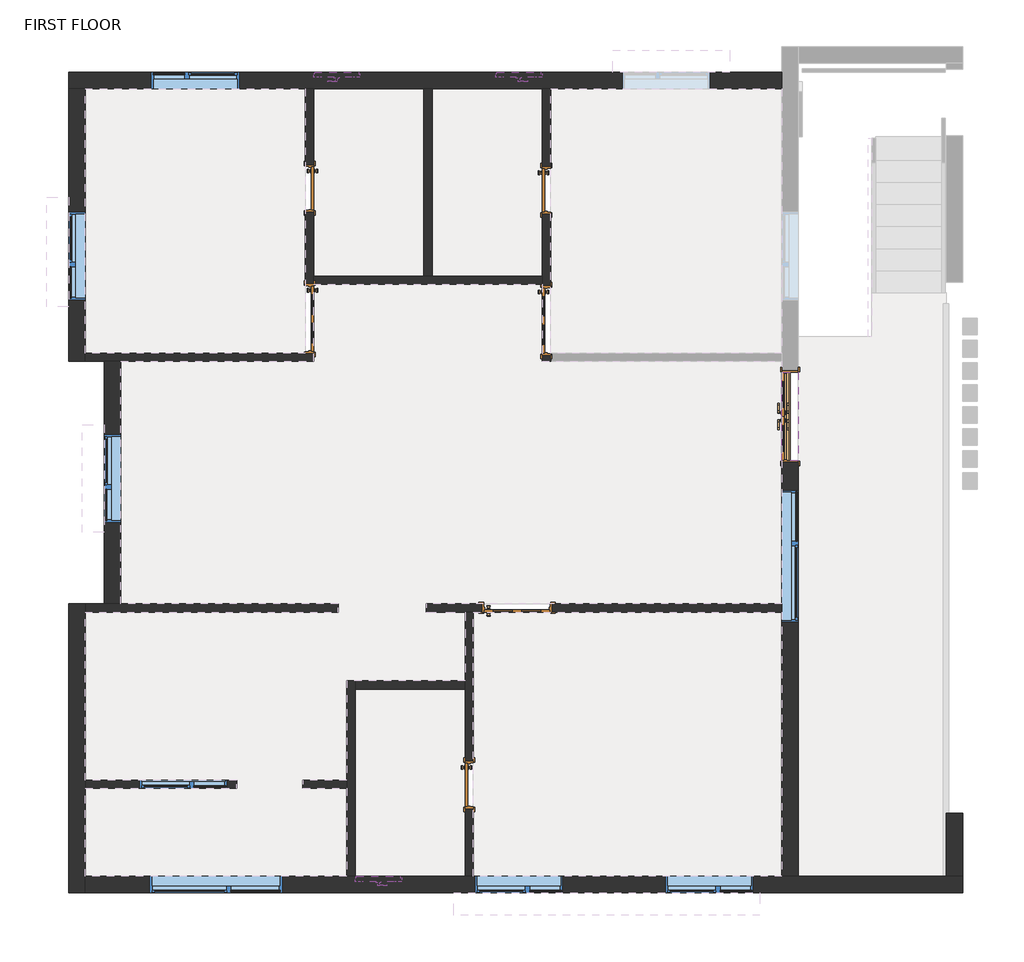
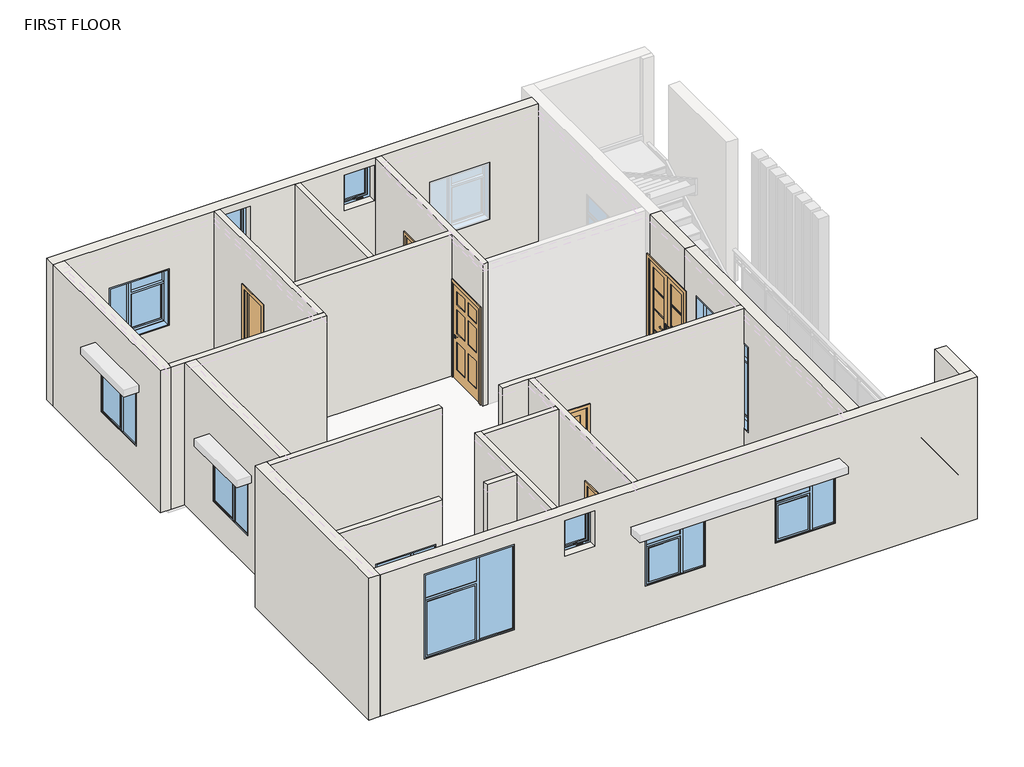
# One storey, part 1 of 2: 20 walls, 11 windows, 7 doors.
"""IFC4 building model written with IfcOpenShell, lengths in millimetres."""

from ifc_helpers import new_model, si_unit, frame, origin, place, context, project, spatial, polyline, outline, extrude, faceted_brep, transform, mapped, element, save
from components import door_exterior_double_full_glass_wood_clad_double_main_door_4_3788f36b, door_92bad2d9, door_a4da38fb, door_0e119d28, door_525aa856, window_610_x_762_5077743b, window_610_x_762_22856471, window_casement_double_sidelight_window_4_x_4_2a492e8f, window_casement_double_sidelight_window_4_x_4_ae1e99d1, window_casement_double_sidelight_window_6_x_6_6a7c62ef

model = new_model("IFC4")

# Units and contexts
model_context = context("Model", 3, world=origin())
ifc_project = project(units=[si_unit("LENGTHUNIT", "METRE", prefix="MILLI")], contexts=[model_context])

# Site, building, storey
site = spatial("IfcSite", under=ifc_project)
building = spatial("IfcBuilding", under=site)
storey = spatial("IfcBuildingStorey", under=building, Name="FIRST FLOOR", Elevation=3048.0)

# Doors
placement = place(None, origin())
door_exterior_double_full_glass_wood_clad_double_main_door_4_shape = door_exterior_double_full_glass_wood_clad_double_main_door_4_3788f36b(model_context)
element("IfcDoor", 1, ObjectType="Door-Exterior-Double-Full Glass-Wood_Clad : double main door 4' x 7'", at=placement, inside=storey, context=model_context, shape_type="MappedRepresentation", body=[
    mapped(door_exterior_double_full_glass_wood_clad_double_main_door_4_shape, transform((-4646.5406154, 1972.1500875, 3022.6), x_axis=(0.0, 1.0, 0.0), y_axis=(-1.0, 0.0, 0.0), z_axis=(0.0, 0.0, 1.0))),
])
door_shape = door_92bad2d9(model_context)
element("IfcDoor", 2, ObjectType="Door-Interior-Single-6_Panel-Wood : 36\" x 80\"", at=placement, inside=storey, context=model_context, shape_type="MappedRepresentation", body=[
    mapped(door_shape, transform((-11288.6406154, 3324.7000875, 3048.0), x_axis=(0.0, -1.0, 0.0), y_axis=(1.0, 0.0, 0.0), z_axis=(0.0, 0.0, 1.0))),
])
door_2_shape = door_a4da38fb(model_context)
element("IfcDoor", 3, ObjectType="Door-Interior-Single-6_Panel-Wood : 36\" x 80\"", at=placement, inside=storey, context=model_context, shape_type="MappedRepresentation", body=[
    mapped(door_2_shape, transform((-8018.3906154, 3299.3000875, 3048.0), x_axis=(0.0, -1.0, 0.0), y_axis=(1.0, 0.0, 0.0), z_axis=(0.0, 0.0, 1.0))),
])
element("IfcDoor", 4, ObjectType="Door-Interior-Single-6_Panel-Wood : 36\" x 80\"", at=placement, inside=storey, context=model_context, shape_type="MappedRepresentation", body=[
    mapped(door_2_shape, transform((-8421.6156154, -678.9749125, 3048.0), x_axis=(1.0, 0.0, 0.0), y_axis=(0.0, 1.0, 0.0), z_axis=(0.0, 0.0, 1.0))),
])
door_3_shape = door_0e119d28(model_context)
element("IfcDoor", 5, ObjectType="Door-Interior-Single-Flush_Panel-Wood : 24\" x 80\"", at=placement, inside=storey, context=model_context, shape_type="MappedRepresentation", body=[
    mapped(door_3_shape, transform((-11288.6406154, 5128.1000875, 3048.0), x_axis=(0.0, -1.0, 0.0), y_axis=(1.0, 0.0, 0.0), z_axis=(0.0, 0.0, 1.0))),
])
door_4_shape = door_525aa856(model_context)
element("IfcDoor", 6, ObjectType="Door-Interior-Single-Flush_Panel-Wood : 24\" x 80\"", at=placement, inside=storey, context=model_context, shape_type="MappedRepresentation", body=[
    mapped(door_4_shape, transform((-8018.3906154, 5102.7000875, 3048.0), x_axis=(0.0, -1.0, 0.0), y_axis=(1.0, 0.0, 0.0), z_axis=(0.0, 0.0, 1.0))),
])
element("IfcDoor", 7, ObjectType="Door-Interior-Single-Flush_Panel-Wood : 24\" x 80\"", at=placement, inside=storey, context=model_context, shape_type="MappedRepresentation", body=[
    mapped(door_4_shape, transform((-9085.1906154, -3123.7249125, 3048.0), x_axis=(0.0, -1.0, 0.0), y_axis=(1.0, 0.0, 0.0), z_axis=(0.0, 0.0, 1.0))),
])

# Walls
element("IfcWall", 8, at=placement, inside=storey, context=model_context, shape_type="Brep", body=[
    faceted_brep([(-4757.6656154, 6734.6500875, 3048.0), (-14625.5656154, 6734.6500875, 3048.0), (-14625.5656154, 6734.6500875, 6096.0), (-4757.6656154, 6734.6500875, 6096.0), (-10612.3656154, 6734.6500875, 5181.6), (-10612.3656154, 6734.6500875, 5943.6), (-11221.9656154, 6734.6500875, 5943.6), (-11221.9656154, 6734.6500875, 5181.6), (-8701.0156154, 6734.6500875, 5943.6), (-8701.0156154, 6734.6500875, 5181.6), (-8091.4156154, 6734.6500875, 5181.6), (-8091.4156154, 6734.6500875, 5943.6), (-5748.2656154, 6734.6500875, 5181.6), (-6967.4656154, 6734.6500875, 5181.6), (-6967.4656154, 6734.6500875, 3962.4), (-5748.2656154, 6734.6500875, 3962.4), (-12263.3656154, 6734.6500875, 5181.6), (-13482.5656154, 6734.6500875, 5181.6), (-13482.5656154, 6734.6500875, 3962.4), (-12263.3656154, 6734.6500875, 3962.4), (-4757.6656154, 6506.0500875, 3048.0), (-4757.6656154, 6506.0500875, 6096.0), (-7958.0656154, 6506.0500875, 6096.0), (-8072.3656154, 6506.0500875, 6096.0), (-9596.3656154, 6506.0500875, 6096.0), (-9710.6656154, 6506.0500875, 6096.0), (-11234.6656154, 6506.0500875, 6096.0), (-11348.9656154, 6506.0500875, 6096.0), (-14396.9656154, 6506.0500875, 6096.0), (-14625.5656154, 6506.0500875, 6096.0), (-14625.5656154, 6506.0500875, 3048.0), (-14396.9656154, 6506.0500875, 3048.0), (-11348.9656154, 6506.0500875, 3048.0), (-11234.6656154, 6506.0500875, 3048.0), (-9710.6656154, 6506.0500875, 3048.0), (-9596.3656154, 6506.0500875, 3048.0), (-8072.3656154, 6506.0500875, 3048.0), (-7958.0656154, 6506.0500875, 3048.0), (-10612.3656154, 6506.0500875, 5943.6), (-10612.3656154, 6506.0500875, 5181.6), (-11221.9656154, 6506.0500875, 5181.6), (-11221.9656154, 6506.0500875, 5943.6), (-8701.0156154, 6506.0500875, 5181.6), (-8701.0156154, 6506.0500875, 5943.6), (-8091.4156154, 6506.0500875, 5943.6), (-8091.4156154, 6506.0500875, 5181.6), (-5748.2656154, 6506.0500875, 5181.6), (-5748.2656154, 6506.0500875, 3962.4), (-6967.4656154, 6506.0500875, 3962.4), (-6967.4656154, 6506.0500875, 5181.6), (-12263.3656154, 6506.0500875, 5181.6), (-12263.3656154, 6506.0500875, 3962.4), (-13482.5656154, 6506.0500875, 3962.4), (-13482.5656154, 6506.0500875, 5181.6)], [[[0, 1, 2, 3], [4, 5, 6, 7], [8, 9, 10, 11], [12, 13, 14, 15], [16, 17, 18, 19]], [[20, 21, 22, 23, 24, 25, 26, 27, 28, 29, 30, 31, 32, 33, 34, 35, 36, 37], [38, 39, 40, 41], [42, 43, 44, 45], [46, 47, 48, 49], [50, 51, 52, 53]], [[1, 0, 20, 37, 36, 35, 34, 33, 32, 31, 30]], [[3, 2, 29, 28, 27, 26, 25, 24, 23, 22, 21]], [[2, 1, 30, 29]], [[39, 38, 5, 4]], [[4, 7, 40, 39]], [[7, 6, 41, 40]], [[38, 41, 6, 5]], [[42, 9, 8, 43]], [[9, 42, 45, 10]], [[10, 45, 44, 11]], [[43, 8, 11, 44]], [[47, 46, 12, 15]], [[48, 47, 15, 14]], [[49, 48, 14, 13]], [[46, 49, 13, 12]], [[51, 50, 16, 19]], [[52, 51, 19, 18]], [[53, 52, 18, 17]], [[50, 53, 17, 16]], [[0, 3, 21, 20]]]),
])
element("IfcWall", 9, at=placement, inside=storey, context=model_context, shape_type="Brep", body=[
    faceted_brep([(-14625.5656154, 6506.0500875, 3048.0), (-14625.5656154, 2734.1500875, 3048.0), (-14625.5656154, 2734.1500875, 6096.0), (-14625.5656154, 6506.0500875, 6096.0), (-14625.5656154, 4803.1295492, 5181.6), (-14625.5656154, 3583.9295492, 5181.6), (-14625.5656154, 3583.9295492, 3962.4), (-14625.5656154, 4803.1295492, 3962.4), (-14396.9656154, 6506.0500875, 3048.0), (-14396.9656154, 6506.0500875, 6096.0), (-14396.9656154, 2848.4500875, 6096.0), (-14396.9656154, 2734.1500875, 6096.0), (-14396.9656154, 2734.1500875, 3048.0), (-14396.9656154, 2848.4500875, 3048.0), (-14396.9656154, 4803.1295492, 5181.6), (-14396.9656154, 4803.1295492, 3962.4), (-14396.9656154, 3583.9295492, 3962.4), (-14396.9656154, 3583.9295492, 5181.6)], [[[0, 1, 2, 3], [4, 5, 6, 7]], [[8, 9, 10, 11, 12, 13], [14, 15, 16, 17]], [[1, 0, 8, 13, 12]], [[3, 2, 11, 10, 9]], [[0, 3, 9, 8]], [[2, 1, 12, 11]], [[15, 14, 4, 7]], [[16, 15, 7, 6]], [[17, 16, 6, 5]], [[14, 17, 5, 4]]]),
])
element("IfcWall", 10, at=placement, inside=storey, context=model_context, shape_type="Brep", body=[
    faceted_brep([(-14625.5656154, -618.6499125, 3048.0), (-14625.5656154, -4619.1499125, 3048.0), (-14625.5656154, -4619.1499125, 6096.0), (-14625.5656154, -618.6499125, 6096.0), (-14396.9656154, -618.6499125, 3048.0), (-14396.9656154, -618.6499125, 6096.0), (-14396.9656154, -732.9499125, 6096.0), (-14396.9656154, -3057.0499125, 6096.0), (-14396.9656154, -3171.3499125, 6096.0), (-14396.9656154, -4390.5499125, 6096.0), (-14396.9656154, -4619.1499125, 6096.0), (-14396.9656154, -4619.1499125, 3048.0), (-14396.9656154, -4390.5499125, 3048.0), (-14396.9656154, -3171.3499125, 3048.0), (-14396.9656154, -3057.0499125, 3048.0), (-14396.9656154, -732.9499125, 3048.0)], [[[0, 1, 2, 3]], [[4, 5, 6, 7, 8, 9, 10, 11, 12, 13, 14, 15]], [[1, 0, 4, 15, 14, 13, 12, 11]], [[3, 2, 10, 9, 8, 7, 6, 5]], [[2, 1, 11, 10]], [[0, 3, 5, 4]]]),
])
element("IfcWall", 11, at=placement, inside=storey, context=model_context, shape_type="Brep", body=[
    faceted_brep([(-14396.9656154, -4619.1499125, 3048.0), (-2255.7656154, -4619.1499125, 3048.0), (-2255.7656154, -4619.1499125, 6096.0), (-14396.9656154, -4619.1499125, 6096.0), (-10644.1156154, -4619.1499125, 5181.6), (-10644.1156154, -4619.1499125, 5943.6), (-10034.5156154, -4619.1499125, 5943.6), (-10034.5156154, -4619.1499125, 5181.6), (-9005.8156154, -4619.1499125, 5181.6), (-7786.6156154, -4619.1499125, 5181.6), (-7786.6156154, -4619.1499125, 3962.4), (-9005.8156154, -4619.1499125, 3962.4), (-6370.5656154, -4619.1499125, 5181.6), (-5151.3656154, -4619.1499125, 5181.6), (-5151.3656154, -4619.1499125, 3962.4), (-6370.5656154, -4619.1499125, 3962.4), (-13501.6156154, -4619.1499125, 5791.2), (-11672.8156154, -4619.1499125, 5791.2), (-11672.8156154, -4619.1499125, 3962.4), (-13501.6156154, -4619.1499125, 3962.4), (-14396.9656154, -4390.5499125, 3048.0), (-14396.9656154, -4390.5499125, 6096.0), (-10777.4656154, -4390.5499125, 6096.0), (-10663.1656154, -4390.5499125, 6096.0), (-9139.1656154, -4390.5499125, 6096.0), (-9024.8656154, -4390.5499125, 6096.0), (-4757.6656154, -4390.5499125, 6096.0), (-4529.0656154, -4390.5499125, 6096.0), (-2484.3656154, -4390.5499125, 6096.0), (-2255.7656154, -4390.5499125, 6096.0), (-2255.7656154, -4390.5499125, 3048.0), (-2484.3656154, -4390.5499125, 3048.0), (-4529.0656154, -4390.5499125, 3048.0), (-4757.6656154, -4390.5499125, 3048.0), (-9024.8656154, -4390.5499125, 3048.0), (-9139.1656154, -4390.5499125, 3048.0), (-10663.1656154, -4390.5499125, 3048.0), (-10777.4656154, -4390.5499125, 3048.0), (-10644.1156154, -4390.5499125, 5943.6), (-10644.1156154, -4390.5499125, 5181.6), (-10034.5156154, -4390.5499125, 5181.6), (-10034.5156154, -4390.5499125, 5943.6), (-9005.8156154, -4390.5499125, 5181.6), (-9005.8156154, -4390.5499125, 3962.4), (-7786.6156154, -4390.5499125, 3962.4), (-7786.6156154, -4390.5499125, 5181.6), (-6370.5656154, -4390.5499125, 5181.6), (-6370.5656154, -4390.5499125, 3962.4), (-5151.3656154, -4390.5499125, 3962.4), (-5151.3656154, -4390.5499125, 5181.6), (-13501.6156154, -4390.5499125, 5791.2), (-13501.6156154, -4390.5499125, 3962.4), (-11672.8156154, -4390.5499125, 3962.4), (-11672.8156154, -4390.5499125, 5791.2)], [[[0, 1, 2, 3], [4, 5, 6, 7], [8, 9, 10, 11], [12, 13, 14, 15], [16, 17, 18, 19]], [[20, 21, 22, 23, 24, 25, 26, 27, 28, 29, 30, 31, 32, 33, 34, 35, 36, 37], [38, 39, 40, 41], [42, 43, 44, 45], [46, 47, 48, 49], [50, 51, 52, 53]], [[1, 0, 20, 37, 36, 35, 34, 33, 32, 31, 30]], [[3, 2, 29, 28, 27, 26, 25, 24, 23, 22, 21]], [[0, 3, 21, 20]], [[4, 39, 38, 5]], [[39, 4, 7, 40]], [[40, 7, 6, 41]], [[5, 38, 41, 6]], [[43, 42, 8, 11]], [[44, 43, 11, 10]], [[45, 44, 10, 9]], [[42, 45, 9, 8]], [[47, 46, 12, 15]], [[48, 47, 15, 14]], [[49, 48, 14, 13]], [[46, 49, 13, 12]], [[51, 50, 16, 19]], [[52, 51, 19, 18]], [[53, 52, 18, 17]], [[50, 53, 17, 16]], [[2, 1, 30, 29]]]),
])
element("IfcWall", 12, at=placement, inside=storey, context=model_context, shape_type="Brep", body=[
    faceted_brep([(-4529.0656154, 1362.5500875, 6096.0), (-4529.0656154, -4390.5499125, 6096.0), (-4529.0656154, -4390.5499125, 3048.0), (-4529.0656154, 1337.1500875, 3048.0), (-4529.0656154, 1337.1500875, 5181.6), (-4529.0656154, 1362.5500875, 5181.6), (-4529.0656154, -875.0434232, 5334.0), (-4529.0656154, 953.7565768, 5334.0), (-4529.0656154, 953.7565768, 3505.2), (-4529.0656154, -875.0434232, 3505.2), (-4757.6656154, -4390.5499125, 6096.0), (-4757.6656154, -732.9499125, 6096.0), (-4757.6656154, -618.6499125, 6096.0), (-4757.6656154, 1362.5500875, 6096.0), (-4757.6656154, 1362.5500875, 5181.6), (-4757.6656154, 1337.1500875, 5181.6), (-4757.6656154, 1337.1500875, 3048.0), (-4757.6656154, -618.6499125, 3048.0), (-4757.6656154, -732.9499125, 3048.0), (-4757.6656154, -4390.5499125, 3048.0), (-4757.6656154, -875.0434232, 5334.0), (-4757.6656154, -875.0434232, 3505.2), (-4757.6656154, 953.7565768, 3505.2), (-4757.6656154, 953.7565768, 5334.0)], [[[0, 1, 2, 3, 4, 5], [6, 7, 8, 9]], [[10, 11, 12, 13, 14, 15, 16, 17, 18, 19], [20, 21, 22, 23]], [[2, 19, 18, 17, 16, 3]], [[13, 0, 5, 14]], [[1, 0, 13, 12, 11, 10]], [[2, 1, 10, 19]], [[4, 15, 14, 5]], [[15, 4, 3, 16]], [[21, 20, 6, 9]], [[22, 21, 9, 8]], [[23, 22, 8, 7]], [[20, 23, 7, 6]]]),
])
element("IfcWall", 13, at=placement, inside=storey, context=model_context, shape_type="Brep", body=[
    faceted_brep([(-14396.9656154, -732.9499125, 3048.0), (-10895.4913348, -732.9499125, 3048.0), (-10895.4913348, -732.9499125, 6096.0), (-14396.9656154, -732.9499125, 6096.0), (-14396.9656154, -618.6499125, 3048.0), (-14396.9656154, -618.6499125, 6096.0), (-14130.2656154, -618.6499125, 6096.0), (-13901.6656154, -618.6499125, 6096.0), (-10895.4913348, -618.6499125, 6096.0), (-10895.4913348, -618.6499125, 3048.0), (-13901.6656154, -618.6499125, 3048.0), (-14130.2656154, -618.6499125, 3048.0)], [[[0, 1, 2, 3]], [[4, 5, 6, 7, 8, 9, 10, 11]], [[1, 0, 4, 11, 10, 9]], [[2, 1, 9, 8]], [[3, 2, 8, 7, 6, 5]], [[0, 3, 5, 4]]]),
])
element("IfcWall", 14, at=placement, inside=storey, context=model_context, shape_type="SweptSolid", body=[
    extrude(outline(polyline([(3048.0, -14396.9656154), (3048.0, -12301.4656154), (6096.0, -12301.4656154), (6096.0, -14396.9656154), (3048.0, -14396.9656154)]), holes=[polyline([(5181.6, -13647.6656154), (5181.6, -12428.4656154), (3962.4, -12428.4656154), (3962.4, -13647.6656154), (5181.6, -13647.6656154)])]), frame((0.0, -3171.3499125, 0.0), z_axis=(0.0, 1.0, 0.0), x_axis=(0.0, 0.0, 1.0)), (0.0, 0.0, 1.0), 114.3),
])
element("IfcWall", 15, at=placement, inside=storey, context=model_context, shape_type="SweptSolid", body=[
    extrude(outline(polyline([(-11387.0656154, -3057.0499125), (-10777.4656154, -3057.0499125), (-10777.4656154, -3171.3499125), (-11387.0656154, -3171.3499125), (-11387.0656154, -3057.0499125)])), frame((0.0, 0.0, 3048.0), z_axis=(0.0, 0.0, 1.0), x_axis=(1.0, 0.0, 0.0)), (0.0, 0.0, 1.0), 3048.0),
])
element("IfcWall", 16, at=placement, inside=storey, context=model_context, shape_type="Brep", body=[
    faceted_brep([(-10663.1656154, -4390.5499125, 3048.0), (-10663.1656154, -1799.7499125, 3048.0), (-10663.1656154, -1685.4499125, 3048.0), (-10663.1656154, -1685.4499125, 6096.0), (-10663.1656154, -1799.7499125, 6096.0), (-10663.1656154, -4390.5499125, 6096.0), (-10777.4656154, -4390.5499125, 3048.0), (-10777.4656154, -4390.5499125, 6096.0), (-10777.4656154, -3171.3499125, 6096.0), (-10777.4656154, -3057.0499125, 6096.0), (-10777.4656154, -1685.4499125, 6096.0), (-10777.4656154, -1685.4499125, 3048.0), (-10777.4656154, -3057.0499125, 3048.0), (-10777.4656154, -3171.3499125, 3048.0)], [[[0, 1, 2, 3, 4, 5]], [[6, 7, 8, 9, 10, 11, 12, 13]], [[2, 1, 0, 6, 13, 12, 11]], [[5, 4, 3, 10, 9, 8, 7]], [[0, 5, 7, 6]], [[3, 2, 11, 10]]]),
])
element("IfcWall", 17, at=placement, inside=storey, context=model_context, shape_type="SweptSolid", body=[
    extrude(outline(polyline([(-9139.1656154, -1799.7499125), (-10663.1656154, -1799.7499125), (-10663.1656154, -1685.4499125), (-9139.1656154, -1685.4499125), (-9139.1656154, -1799.7499125)])), frame((0.0, 0.0, 3048.0), z_axis=(0.0, 0.0, 1.0), x_axis=(1.0, 0.0, 0.0)), (0.0, 0.0, 1.0), 3048.0),
])
element("IfcWall", 18, at=placement, inside=storey, context=model_context, shape_type="Brep", body=[
    faceted_brep([(-9024.8656154, -732.9499125, 6096.0), (-9024.8656154, -4390.5499125, 6096.0), (-9024.8656154, -4390.5499125, 3048.0), (-9024.8656154, -3453.9249125, 3048.0), (-9024.8656154, -3453.9249125, 5105.4), (-9024.8656154, -2793.5249125, 5105.4), (-9024.8656154, -2793.5249125, 3048.0), (-9024.8656154, -732.9499125, 3048.0), (-9139.1656154, -4390.5499125, 6096.0), (-9139.1656154, -1799.7499125, 6096.0), (-9139.1656154, -1685.4499125, 6096.0), (-9139.1656154, -732.9499125, 6096.0), (-9139.1656154, -732.9499125, 3048.0), (-9139.1656154, -1685.4499125, 3048.0), (-9139.1656154, -1799.7499125, 3048.0), (-9139.1656154, -2793.5249125, 3048.0), (-9139.1656154, -2793.5249125, 5105.4), (-9139.1656154, -3453.9249125, 5105.4), (-9139.1656154, -3453.9249125, 3048.0), (-9139.1656154, -4390.5499125, 3048.0)], [[[0, 1, 2, 3, 4, 5, 6, 7]], [[8, 9, 10, 11, 12, 13, 14, 15, 16, 17, 18, 19]], [[12, 7, 6, 15, 14, 13]], [[2, 19, 18, 3]], [[1, 0, 11, 10, 9, 8]], [[0, 7, 12, 11]], [[2, 1, 8, 19]], [[17, 4, 3, 18]], [[4, 17, 16, 5]], [[5, 16, 15, 6]]]),
])
element("IfcWall", 19, at=placement, inside=storey, context=model_context, shape_type="Brep", body=[
    faceted_brep([(-8072.3656154, 2734.1500875, 6096.0), (-8072.3656154, 3800.9500875, 6096.0), (-8072.3656154, 3915.2500875, 6096.0), (-8072.3656154, 6506.0500875, 6096.0), (-8072.3656154, 6506.0500875, 3048.0), (-8072.3656154, 5432.9000875, 3048.0), (-8072.3656154, 5432.9000875, 5105.4), (-8072.3656154, 4772.5000875, 5105.4), (-8072.3656154, 4772.5000875, 3048.0), (-8072.3656154, 3915.2500875, 3048.0), (-8072.3656154, 3800.9500875, 3048.0), (-8072.3656154, 3781.9000875, 3048.0), (-8072.3656154, 3781.9000875, 5105.4), (-8072.3656154, 2816.7000875, 5105.4), (-8072.3656154, 2816.7000875, 3048.0), (-8072.3656154, 2734.1500875, 3048.0), (-7958.0656154, 6506.0500875, 6096.0), (-7958.0656154, 2848.4500875, 6096.0), (-7958.0656154, 2734.1500875, 6096.0), (-7958.0656154, 2734.1500875, 3048.0), (-7958.0656154, 2816.7000875, 3048.0), (-7958.0656154, 2816.7000875, 5105.4), (-7958.0656154, 3781.9000875, 5105.4), (-7958.0656154, 3781.9000875, 3048.0), (-7958.0656154, 4772.5000875, 3048.0), (-7958.0656154, 4772.5000875, 5105.4), (-7958.0656154, 5432.9000875, 5105.4), (-7958.0656154, 5432.9000875, 3048.0), (-7958.0656154, 6506.0500875, 3048.0)], [[[0, 1, 2, 3, 4, 5, 6, 7, 8, 9, 10, 11, 12, 13, 14, 15]], [[16, 17, 18, 19, 20, 21, 22, 23, 24, 25, 26, 27, 28]], [[4, 28, 27, 5]], [[19, 15, 14, 20]], [[23, 11, 10, 9, 8, 24]], [[3, 2, 1, 0, 18, 17, 16]], [[4, 3, 16, 28]], [[0, 15, 19, 18]], [[14, 13, 21, 20]], [[13, 12, 22, 21]], [[12, 11, 23, 22]], [[7, 25, 24, 8]], [[25, 7, 6, 26]], [[26, 6, 5, 27]]]),
])
element("IfcWall", 20, at=placement, inside=storey, context=model_context, shape_type="Brep", body=[
    faceted_brep([(-8072.3656154, 3915.2500875, 3048.0), (-9596.3656154, 3915.2500875, 3048.0), (-9710.6656154, 3915.2500875, 3048.0), (-11234.6656154, 3915.2500875, 3048.0), (-11234.6656154, 3915.2500875, 6096.0), (-9710.6656154, 3915.2500875, 6096.0), (-9596.3656154, 3915.2500875, 6096.0), (-8072.3656154, 3915.2500875, 6096.0), (-8072.3656154, 3800.9500875, 3048.0), (-8072.3656154, 3800.9500875, 6096.0), (-11234.6656154, 3800.9500875, 6096.0), (-11234.6656154, 3800.9500875, 3048.0), (-11234.6656154, 3807.3000875, 3048.0)], [[[0, 1, 2, 3, 4, 5, 6, 7]], [[8, 9, 10, 11]], [[3, 2, 1, 0, 8, 11, 12]], [[7, 6, 5, 4, 10, 9]], [[0, 7, 9, 8]], [[4, 3, 12, 11, 10]]]),
])
element("IfcWall", 21, at=placement, inside=storey, context=model_context, shape_type="Brep", body=[
    faceted_brep([(-11234.6656154, 6506.0500875, 6096.0), (-11234.6656154, 3915.2500875, 6096.0), (-11234.6656154, 3800.9500875, 6096.0), (-11234.6656154, 2848.4500875, 6096.0), (-11234.6656154, 2848.4500875, 5105.4), (-11234.6656154, 3807.3000875, 5105.4), (-11234.6656154, 3807.3000875, 3048.0), (-11234.6656154, 3915.2500875, 3048.0), (-11234.6656154, 4797.9000875, 3048.0), (-11234.6656154, 4797.9000875, 5105.4), (-11234.6656154, 5458.3000875, 5105.4), (-11234.6656154, 5458.3000875, 3048.0), (-11234.6656154, 6506.0500875, 3048.0), (-11348.9656154, 2848.4500875, 6096.0), (-11348.9656154, 6506.0500875, 6096.0), (-11348.9656154, 6506.0500875, 3048.0), (-11348.9656154, 5458.3000875, 3048.0), (-11348.9656154, 5458.3000875, 5105.4), (-11348.9656154, 4797.9000875, 5105.4), (-11348.9656154, 4797.9000875, 3048.0), (-11348.9656154, 3807.3000875, 3048.0), (-11348.9656154, 3807.3000875, 5105.4), (-11348.9656154, 2848.4500875, 5105.4)], [[[0, 1, 2, 3, 4, 5, 6, 7, 8, 9, 10, 11, 12]], [[13, 14, 15, 16, 17, 18, 19, 20, 21, 22]], [[15, 12, 11, 16]], [[6, 20, 19, 8, 7]], [[3, 2, 1, 0, 14, 13]], [[0, 12, 15, 14]], [[3, 13, 22, 4]], [[21, 5, 4, 22]], [[5, 21, 20, 6]], [[18, 9, 8, 19]], [[9, 18, 17, 10]], [[10, 17, 16, 11]]]),
])
element("IfcWall", 22, at=placement, inside=storey, context=model_context, shape_type="SweptSolid", body=[
    extrude(outline(polyline([(-9710.6656154, 3915.2500875), (-9710.6656154, 6506.0500875), (-9596.3656154, 6506.0500875), (-9596.3656154, 3915.2500875), (-9710.6656154, 3915.2500875)])), frame((0.0, 0.0, 3048.0), z_axis=(0.0, 0.0, 1.0), x_axis=(1.0, 0.0, 0.0)), (0.0, 0.0, 1.0), 3048.0),
])
element("IfcWall", 23, at=placement, inside=storey, context=model_context, shape_type="Brep", body=[
    faceted_brep([(-14396.9656154, 2734.1500875, 3048.0), (-14130.2656154, 2734.1500875, 3048.0), (-13901.6656154, 2734.1500875, 3048.0), (-11234.6656154, 2734.1500875, 3048.0), (-11234.6656154, 2734.1500875, 6096.0), (-13901.6656154, 2734.1500875, 6096.0), (-14130.2656154, 2734.1500875, 6096.0), (-14396.9656154, 2734.1500875, 6096.0), (-14396.9656154, 2848.4500875, 6096.0), (-11348.9656154, 2848.4500875, 6096.0), (-11234.6656154, 2848.4500875, 6096.0), (-11234.6656154, 2848.4500875, 5105.4), (-11348.9656154, 2848.4500875, 5105.4), (-11348.9656154, 2848.4500875, 3048.0), (-14396.9656154, 2848.4500875, 3048.0), (-11348.9656154, 2842.1000875, 3048.0), (-11234.6656154, 2842.1000875, 3048.0), (-11234.6656154, 2842.1000875, 5105.4), (-11348.9656154, 2842.1000875, 5105.4)], [[[0, 1, 2, 3, 4, 5, 6, 7]], [[8, 9, 10, 11, 12, 13, 14]], [[3, 2, 1, 0, 14, 13, 15, 16]], [[7, 6, 5, 4, 10, 9, 8]], [[0, 7, 8, 14]], [[4, 3, 16, 17, 11, 10]], [[18, 15, 13, 12]], [[15, 18, 17, 16]], [[17, 18, 12, 11]]]),
])
element("IfcWall", 24, at=placement, inside=storey, context=model_context, shape_type="SweptSolid", body=[
    extrude(outline(polyline([(-4757.6656154, 1362.5500875), (-4757.6656154, 2581.7500875), (-4529.0656154, 2581.7500875), (-4529.0656154, 1362.5500875), (-4757.6656154, 1362.5500875)])), frame((0.0, 0.0, 5181.6), z_axis=(0.0, 0.0, 1.0), x_axis=(1.0, 0.0, 0.0)), (0.0, 0.0, 1.0), 914.4),
])
element("IfcWall", 25, at=placement, inside=storey, context=model_context, shape_type="Brep", body=[
    faceted_brep([(-9676.2913348, -618.6499125, 3048.0), (-9676.2913348, -618.6499125, 6096.0), (-4757.6656154, -618.6499125, 6096.0), (-4757.6656154, -618.6499125, 3048.0), (-7939.0156154, -618.6499125, 3048.0), (-7939.0156154, -618.6499125, 5105.4), (-8904.2156154, -618.6499125, 5105.4), (-8904.2156154, -618.6499125, 3048.0), (-9676.2913348, -732.9499125, 6096.0), (-9676.2913348, -732.9499125, 3048.0), (-9139.1656154, -732.9499125, 3048.0), (-9024.8656154, -732.9499125, 3048.0), (-8904.2156154, -732.9499125, 3048.0), (-8904.2156154, -732.9499125, 5105.4), (-7939.0156154, -732.9499125, 5105.4), (-7939.0156154, -732.9499125, 3048.0), (-4757.6656154, -732.9499125, 3048.0), (-4757.6656154, -732.9499125, 6096.0), (-9024.8656154, -732.9499125, 6096.0), (-9139.1656154, -732.9499125, 6096.0)], [[[0, 1, 2, 3, 4, 5, 6, 7]], [[8, 9, 10, 11, 12, 13, 14, 15, 16, 17, 18, 19]], [[9, 0, 7, 12, 11, 10]], [[3, 16, 15, 4]], [[1, 0, 9, 8]], [[2, 1, 8, 19, 18, 17]], [[3, 2, 17, 16]], [[14, 5, 4, 15]], [[5, 14, 13, 6]], [[6, 13, 12, 7]]]),
])
element("IfcWall", 26, at=placement, inside=storey, context=model_context, shape_type="SweptSolid", body=[
    extrude(outline(polyline([(2734.1500875, 3048.0), (-618.6499125, 3048.0), (-618.6499125, 6096.0), (2734.1500875, 6096.0), (2734.1500875, 3048.0)]), holes=[polyline([(1724.5000875, 4948.6955341), (505.3000875, 4948.6955341), (505.3000875, 3729.4955341), (1724.5000875, 3729.4955341), (1724.5000875, 4948.6955341)])]), frame((-14130.2656154, 0.0, 0.0), z_axis=(1.0, 0.0, 0.0), x_axis=(0.0, 1.0, 0.0)), (0.0, 0.0, 1.0), 228.6),
])
element("IfcWall", 27, at=placement, inside=storey, context=model_context, shape_type="SweptSolid", body=[
    extrude(outline(polyline([(-2255.7656154, -3514.2499125), (-2255.7656154, -4390.5499125), (-2484.3656154, -4390.5499125), (-2484.3656154, -3514.2499125), (-2255.7656154, -3514.2499125)])), frame((0.0, 0.0, 3048.0), z_axis=(0.0, 0.0, 1.0), x_axis=(1.0, 0.0, 0.0)), (0.0, 0.0, 1.0), 3048.0),
])

# Windows
window_610_x_762_shape = window_610_x_762_5077743b(model_context)
element("IfcWindow", 28, ObjectType="610 x 762", at=placement, inside=storey, context=model_context, shape_type="MappedRepresentation", body=[
    mapped(window_610_x_762_shape, transform((-10917.1656154, 6620.3500875, 4381.6), x_axis=(-1.0, 0.0, 0.0), y_axis=(0.0, -1.0, 0.0), z_axis=(0.0, 0.0, 1.0))),
])
window_610_x_762_2_shape = window_610_x_762_22856471(model_context)
element("IfcWindow", 29, ObjectType="610 x 762", at=placement, inside=storey, context=model_context, shape_type="MappedRepresentation", body=[
    mapped(window_610_x_762_2_shape, transform((-8396.2156154, 6620.3500875, 4381.6), x_axis=(1.0, 0.0, 0.0), y_axis=(0.0, 1.0, 0.0), z_axis=(0.0, 0.0, 1.0))),
])
element("IfcWindow", 30, ObjectType="610 x 762", at=placement, inside=storey, context=model_context, shape_type="MappedRepresentation", body=[
    mapped(window_610_x_762_2_shape, transform((-10339.3156154, -4504.8499125, 4381.6), x_axis=(1.0, 0.0, 0.0), y_axis=(0.0, 1.0, 0.0), z_axis=(0.0, 0.0, 1.0))),
])
window_casement_double_sidelight_window_4_x_4_shape = window_casement_double_sidelight_window_4_x_4_2a492e8f(model_context)
element("IfcWindow", 31, ObjectType="Window-Casement-Double-Sidelight : window 4' x 4'", at=placement, inside=storey, context=model_context, shape_type="MappedRepresentation", body=[
    mapped(window_casement_double_sidelight_window_4_x_4_shape, transform((-8396.2156154, -4504.8499125, 3048.0), x_axis=(-1.0, 0.0, 0.0), y_axis=(0.0, -1.0, 0.0), z_axis=(0.0, 0.0, 1.0))),
])
element("IfcWindow", 32, ObjectType="Window-Casement-Double-Sidelight : window 4' x 4'", at=placement, inside=storey, context=model_context, shape_type="MappedRepresentation", body=[
    mapped(window_casement_double_sidelight_window_4_x_4_shape, transform((-5760.9656154, -4504.8499125, 3048.0), x_axis=(-1.0, 0.0, 0.0), y_axis=(0.0, -1.0, 0.0), z_axis=(0.0, 0.0, 1.0))),
])
element("IfcWindow", 33, ObjectType="Window-Casement-Double-Sidelight : window 4' x 4'", at=placement, inside=storey, context=model_context, shape_type="MappedRepresentation", body=[
    mapped(window_casement_double_sidelight_window_4_x_4_shape, transform((-12872.9656154, 6620.3500875, 3048.0), x_axis=(1.0, 0.0, 0.0), y_axis=(0.0, 1.0, 0.0), z_axis=(0.0, 0.0, 1.0))),
])
element("IfcWindow", 34, ObjectType="Window-Casement-Double-Sidelight : window 4' x 4'", at=placement, inside=storey, context=model_context, shape_type="MappedRepresentation", body=[
    mapped(window_casement_double_sidelight_window_4_x_4_shape, transform((-14511.2656154, 4193.5295492, 3048.0), x_axis=(0.0, 1.0, 0.0), y_axis=(-1.0, 0.0, 0.0), z_axis=(0.0, 0.0, 1.0))),
])
element("IfcWindow", 35, ObjectType="Window-Casement-Double-Sidelight : window 4' x 4'", at=placement, inside=storey, context=model_context, shape_type="MappedRepresentation", body=[
    mapped(window_casement_double_sidelight_window_4_x_4_shape, transform((-14015.9656154, 1114.9000875, 2815.0955341), x_axis=(0.0, 1.0, 0.0), y_axis=(-1.0, 0.0, 0.0), z_axis=(0.0, 0.0, 1.0))),
])
window_casement_double_sidelight_window_4_x_4_2_shape = window_casement_double_sidelight_window_4_x_4_ae1e99d1(model_context)
element("IfcWindow", 36, ObjectType="Window-Casement-Double-Sidelight : window 4' x 4'", at=placement, inside=storey, context=model_context, shape_type="MappedRepresentation", body=[
    mapped(window_casement_double_sidelight_window_4_x_4_2_shape, transform((-13038.0656154, -3114.1999125, 3048.0), x_axis=(-1.0, 0.0, 0.0), y_axis=(0.0, -1.0, 0.0), z_axis=(0.0, 0.0, 1.0))),
])
window_casement_double_sidelight_window_6_x_6_shape = window_casement_double_sidelight_window_6_x_6_6a7c62ef(model_context)
element("IfcWindow", 37, ObjectType="Window-Casement-Double-Sidelight : window 6' x 6'", at=placement, inside=storey, context=model_context, shape_type="MappedRepresentation", body=[
    mapped(window_casement_double_sidelight_window_6_x_6_shape, transform((-12587.2156154, -4504.8499125, 3048.0), x_axis=(-1.0, 0.0, 0.0), y_axis=(0.0, -1.0, 0.0), z_axis=(0.0, 0.0, 1.0))),
])
element("IfcWindow", 38, ObjectType="Window-Casement-Double-Sidelight : window 6' x 6'", at=placement, inside=storey, context=model_context, shape_type="MappedRepresentation", body=[
    mapped(window_casement_double_sidelight_window_6_x_6_shape, transform((-4643.3656154, 39.3565768, 2590.8), x_axis=(0.0, -1.0, 0.0), y_axis=(1.0, 0.0, 0.0), z_axis=(0.0, 0.0, 1.0))),
])

save(model, "model.ifc")

# Revit data of these elements
# Type "Door-Exterior-Double-Full Glass-Wood_Clad : double main door 4' x 7'"
#   Type Mark = "14"
#   Assembly Code = "B2030100"
#   Analytic Construction = "French door, wood frame with double glass"
#   Top Rail = 0' - 4 11/16"
#   Threshold Offset [instance default] = 0' - 0 1/2"
#   Thickness = 0' - 1 3/8"
#   Thermal Resistance (R) = 1.9158 (h·ft²·°F)/BTU
#   Swing Angle [instance default] = 90.00°
#   Stiles = 0' - 4 3/4"
#   Rough Width = 4' - 2"
#   Rough Height = 7' - 1"
#   Panel Width = 2' - 0"
#   Door Offset [instance default] = 0' - 0"
#   Height = 7' - 0"
#   Width = 4' - 0"
#   Heat Transfer Coefficient (U) = 0.5220 BTU/(h·ft²·°F)
#   Bottom Rail = 0' - 9 1/8"
#   Exterior Trim [instance default] = yes
#   Threshold [instance default] = yes
#   Show Grill [instance default] = yes
#   Function = 1
#   Trim Material = Cherry
#   Threshold Material = Cherry
#   Panel Material = Cherry
#   Glazing = Glass
#   Frame Material = Cherry
#   Door Handle Material = Aluminum
#   Visual Light Transmittance = 0
#   Solar Heat Gain Coefficient = 0
#   Wall Closure = (empty or 0)
#   Construction Type = (empty or 0)
# Type "Door-Interior-Single-6_Panel-Wood : 36\" x 80\""
#   Type Mark = "9"
#   Assembly Code = "C1020300"
#   Analytic Construction = "Wooden"
#   Top Rail = 0' - 4 11/16"
#   Top Panel = 0' - 11"
#   Thickness = 0' - 1 3/8"
#   Thermal Resistance (R) = 2.5876 (h·ft²·°F)/BTU
#   Swing Angle [instance default] = 90.00°
#   Stiles = 0' - 4 3/4"
#   Rough Width = 3' - 2"
#   Rough Height = 6' - 9"
#   Mullion = 0' - 4 1/2"
#   Lock Rail = 0' - 7 1/2"
#   Intermediate Rail = 0' - 4 1/2"
#   Height = 6' - 8"
#   Width = 3' - 0"
#   Heat Transfer Coefficient (U) = 0.3865 BTU/(h·ft²·°F)
#   Bottom Rail = 0' - 9 1/8"
#   Trim Material = Cherry
#   Panel Material = Cherry
#   Frame Material = Cherry
#   Door Handle Material = Aluminum
#   Visual Light Transmittance = 0
#   Solar Heat Gain Coefficient = 0
#   Wall Closure = (empty or 0)
#   Function = (empty or 0)
# Type "Door-Interior-Single-Flush_Panel-Wood : 24\" x 80\""
#   Type Mark = "12"
#   Assembly Code = "C1020300"
#   Analytic Construction = "Wooden"
#   Thickness = 0' - 1 3/8"
#   Thermal Resistance (R) = 2.5876 (h·ft²·°F)/BTU
#   Swing Angle [instance default] = 90.00°
#   Rough Width = 2' - 2"
#   Rough Height = 6' - 9"
#   Height = 6' - 8"
#   Width = 2' - 0"
#   Heat Transfer Coefficient (U) = 0.3865 BTU/(h·ft²·°F)
#   Trim Material = Cherry
#   Panel Material = Cherry
#   Frame Material = Cherry
#   Door Handle Material = Aluminum
#   Visual Light Transmittance = 0
#   Solar Heat Gain Coefficient = 0
#   Wall Closure = (empty or 0)
#   Function = (empty or 0)
# Type
#   Assembly Code = "B2010"
#   Layers, outside or top first: 0' - 9" "LIGHT BEIGE" (function 1)
# Type
#   Assembly Code = "B2010"
#   Layers, outside or top first: 0' - 4 1/2" "LIGHT BEIGE" (function 1)
# Type "610 x 762"
#   Type Mark = "18"
#   Water resistance = "up to Class E1050, PN-EN 12208:2001"
#   URL = "https://aluprof.com/en/architects/offer/window-and-door-systems/mb-59s-casement-mb-59s-casement-hi"
#   Type IFC Predefined Type = "NOTDEFINED"
#   Resistance to wind load = "up to Class C5, PN-EN 12210:2016"
#   Operation = "SingleTopHungCasement"
#   Opening type = "Top-hung casement opening outwards"
#   Model = "MB-59S Casement"
#   ManufacturerSustainabilityPolicyURL = "https://aluprof.eu/en/company/sustainable-development"
#   Manufacturer = "ALUPROF SA"
#   Keynote = "08511300"
#   IfcExportType = "NOTDEFINED"
#   IfcExportAs = "IfcWindowType"
#   Hardware [instance default] = ""
#   Handle type [instance default] = ""
#   Glazing construction = "4/16/4"
#   Export Type to IFC As = "IfcWindowType"
#   Description = "Single top-hung casement opening outwards"
#   Content of the recyclate in the material = "69.2%"
#   COBie.Type.Name = "MB-59S Casement"
#   COBie.Type.Manufacturer = "ALUPROF SA\r\nALUPROF S.A.\r\nALUPROF S.A."
#   Assembly Code = "B2020110"
#   Analytic Construction = "<None>"
#   Air permeability = "up to Class 4, PN-EN 12207:2001"
#   Thermal insulation = 0.299387 BTU/(h·ft²·°F)
#   Sash thickness = 0' - 2.32283"
#   Rough Width = 2' - 1.1811"
#   Rough Height = 2' - 7.1811"
#   Reference line height [instance default] = 0' - 0"
#   Opening angle [instance default] = 0.00°
#   Mounting space = 0' - 0.59055"
#   Height = 2' - 6"
#   Glazing area = 2.82349 SF
#   Frame thickness = 0' - 1.9685"
#   Exterior wall face offset = 0' - 0.7874"
#   Sill Height = 2' - 7.49606"
#   Width = 2' - 0"
#   Warm installation [instance default] = yes
#   Thermal variant HI = no
#   Schedule No. [instance default] = 1
#   IsWindowOpen [instance default] = no
#   IsExternal = yes
#   Define Thermal Properties by = 1
#   COBie.Type = yes
#   COBie = yes
#   Wall Closure = (empty or 0)
# Type "Window-Casement-Double-Sidelight : window 4' x 4'"
#   Type Mark = "22"
#   Fire Rating = "0.5h"
#   Assembly Code = "B2020100"
#   Analytic Construction = "Double glazing - domestic"
#   Window Inset [instance default] = 0' - 0 5/8"
#   Wall Thickness [instance default] = 0' - 6"
#   Visual Light Transmittance = 0.81
#   Transom Height Ratio = 0.3
#   Transom Height = 1' - 2.4"
#   Thermal Resistance (R) = 1.8146 (h·ft²·°F)/BTU
#   Solar Heat Gain Coefficient = 0.76
#   Side Width = 1' - 7.2"
#   Rough Width = 4' - 0 1/2"
#   Rough Height = 4' - 0 1/2"
#   Opening Window Width = 2' - 4.8"
#   Opening Window Height = 2' - 9.6"
#   Heat Transfer Coefficient (U) = 0.5511 BTU/(h·ft²·°F)
#   Height = 4' - 0"
#   Frame Gap 3 [instance default] = 0' - 1 83/128"
#   Frame Gap 2 [instance default] = 0' - 0 5/8"
#   Frame Gap 1 = 0' - 1 51/128"
#   Default Sill Height = 3' - 0"
#   Width = 4' - 0"
#   Frame Material = Metal - Aluminum
#   Glass Panel Material = Glass
#   Wall Closure = (empty or 0)
# Type "Window-Casement-Double-Sidelight : window 6' x 6'"
#   Type Mark = "23"
#   Fire Rating = "0.5h"
#   Assembly Code = "B2020100"
#   Analytic Construction = "Double glazing - domestic"
#   Window Inset [instance default] = 0' - 0 5/8"
#   Wall Thickness [instance default] = 0' - 6"
#   Visual Light Transmittance = 0.81
#   Transom Height Ratio = 0.3
#   Transom Height = 1' - 9.6"
#   Thermal Resistance (R) = 1.8146 (h·ft²·°F)/BTU
#   Solar Heat Gain Coefficient = 0.76
#   Side Width = 2' - 4.8"
#   Rough Width = 6' - 0 1/2"
#   Rough Height = 6' - 0 1/2"
#   Opening Window Width = 3' - 7.2"
#   Opening Window Height = 4' - 2.4"
#   Heat Transfer Coefficient (U) = 0.5511 BTU/(h·ft²·°F)
#   Height = 6' - 0"
#   Frame Gap 3 [instance default] = 0' - 1 83/128"
#   Frame Gap 2 [instance default] = 0' - 0 5/8"
#   Frame Gap 1 = 0' - 1 51/128"
#   Default Sill Height = 3' - 0"
#   Width = 6' - 0"
#   Frame Material = Metal - Aluminum
#   Glass Panel Material = Glass
#   Wall Closure = (empty or 0)
# Element 1 (IfcDoor, "Door-Exterior-Double-Full Glass-Wood_Clad : double main door 4' x 7'")
#   Threshold Offset = 0' - 0 1/2"
#   Swing Angle = 90.00°
#   Door Offset = 0' - 0"
#   Threshold = yes
#   Show Grill = yes
#   Exterior Trim = yes
#   Phase Created = New Construction
#   Materials on its faces: "Cherry", "Aluminum", "Glass"
# Elements 2, 3, 4 (IfcDoor, "Door-Interior-Single-6_Panel-Wood : 36\" x 80\"")
#   Swing Angle = 90.00°
#   Phase Created = New Construction
#   Materials on its faces: "Cherry", "Aluminum"
# Elements 5, 6, 7 (IfcDoor, "Door-Interior-Single-Flush_Panel-Wood : 24\" x 80\"")
#   Swing Angle = 90.00°
#   Phase Created = New Construction
#   Materials on its faces: "Cherry", "Aluminum"
# Elements 8, 9, 10, 13, 14, 15, 16, 17, 18, 19, 20, 21, 22, 23, 24, 25, 26 (IfcWall)
#   Top Offset = 0' - 0"
#   Base Offset = 0' - 0"
#   wall height = 10' - 0"
#   Phase Created = New Construction
#   Base Constraint = FIRST FLOOR
#   Top Constraint = SECOND FLR
#   Materials on its faces: "LIGHT BEIGE"
# Elements 11, 27 (IfcWall)
#   Top Offset = 0' - 0"
#   Base Offset = 0' - 0"
#   wall height = 10' - 0"
#   Phase Created = New Construction
#   Base Constraint = FIRST FLOOR
#   Top Constraint = SECOND FLR
#   Materials on its faces: "LIGHT BEIGE", "Concrete, Cast-in-Place gray"
# Element 12 (IfcWall)
#   Top Offset = 0' - 0"
#   Base Offset = 0' - 0"
#   wall height = 10' - 0"
#   Phase Created = New Construction
#   Base Constraint = FIRST FLOOR
#   Top Constraint = SECOND FLR
#   Materials on its faces: "LIGHT BEIGE", "Wood Planks"
# Element 28 (IfcWindow, "610 x 762")
#   Mark = "14"
#   Hardware = ""
#   Handle type = ""
#   Reference line height = 0' - 0"
#   Opening angle = 0.00°
#   Warm installation = yes
#   Schedule No. = 1
#   IsWindowOpen = no
#   Phase Created = New Construction
# Element 29 (IfcWindow, "610 x 762")
#   Mark = "15"
#   Hardware = ""
#   Handle type = ""
#   Reference line height = 0' - 0"
#   Opening angle = 0.00°
#   Warm installation = yes
#   Schedule No. = 1
#   IsWindowOpen = no
#   Phase Created = New Construction
# Element 30 (IfcWindow, "610 x 762")
#   Mark = "16"
#   Hardware = ""
#   Handle type = ""
#   Reference line height = 0' - 0"
#   Opening angle = 0.00°
#   Warm installation = yes
#   Schedule No. = 1
#   IsWindowOpen = no
#   Phase Created = New Construction
# Element 31 (IfcWindow, "Window-Casement-Double-Sidelight : window 4' x 4'")
#   Mark = "17"
#   Window Inset = 0' - 0 5/8"
#   Frame Gap 3 = 0' - 1 83/128"
#   Frame Gap 2 = 0' - 0 5/8"
#   Phase Created = New Construction
#   Materials on its faces: "Metal - Aluminum", "Glass"
# Element 32 (IfcWindow, "Window-Casement-Double-Sidelight : window 4' x 4'")
#   Mark = "18"
#   Window Inset = 0' - 0 5/8"
#   Frame Gap 3 = 0' - 1 83/128"
#   Frame Gap 2 = 0' - 0 5/8"
#   Phase Created = New Construction
#   Materials on its faces: "Metal - Aluminum", "Glass"
# Element 33 (IfcWindow, "Window-Casement-Double-Sidelight : window 4' x 4'")
#   Mark = "24"
#   Window Inset = 0' - 0 5/8"
#   Frame Gap 3 = 0' - 1 83/128"
#   Frame Gap 2 = 0' - 0 5/8"
#   Phase Created = New Construction
#   Materials on its faces: "Metal - Aluminum", "Glass"
# Element 34 (IfcWindow, "Window-Casement-Double-Sidelight : window 4' x 4'")
#   Mark = "25"
#   Window Inset = 0' - 0 5/8"
#   Frame Gap 3 = 0' - 1 83/128"
#   Frame Gap 2 = 0' - 0 5/8"
#   Phase Created = New Construction
#   Materials on its faces: "Metal - Aluminum", "Glass"
# Element 35 (IfcWindow, "Window-Casement-Double-Sidelight : window 4' x 4'")
#   Mark = "28"
#   Window Inset = 0' - 0 5/8"
#   Frame Gap 3 = 0' - 1 83/128"
#   Frame Gap 2 = 0' - 0 5/8"
#   Phase Created = New Construction
#   Materials on its faces: "Metal - Aluminum", "Glass"
# Element 36 (IfcWindow, "Window-Casement-Double-Sidelight : window 4' x 4'")
#   Mark = "20"
#   Window Inset = 0' - 0 5/8"
#   Frame Gap 3 = 0' - 1 83/128"
#   Frame Gap 2 = 0' - 0 5/8"
#   Phase Created = New Construction
#   Materials on its faces: "Metal - Aluminum", "Glass"
# Element 37 (IfcWindow, "Window-Casement-Double-Sidelight : window 6' x 6'")
#   Mark = "19"
#   Window Inset = 0' - 0 5/8"
#   Frame Gap 3 = 0' - 1 83/128"
#   Frame Gap 2 = 0' - 0 5/8"
#   Phase Created = New Construction
#   Materials on its faces: "Metal - Aluminum", "Glass"
# Element 38 (IfcWindow, "Window-Casement-Double-Sidelight : window 6' x 6'")
#   Mark = "22"
#   Window Inset = 0' - 0 5/8"
#   Frame Gap 3 = 0' - 1 83/128"
#   Frame Gap 2 = 0' - 0 5/8"
#   Phase Created = New Construction
#   Materials on its faces: "Metal - Aluminum", "Glass"
# Materials
#   "Cherry": class "Wood", colour RGB 226 177 128, transparency 0, Description = "Prunus Serotina", Cost = 0
#   "Glass": class "Glass", colour RGB 0 128 192, transparency 0.75, Description = "Soda Lime Glass", Cost = 0
#   "Aluminum": class "Metal", colour RGB 247 247 247, transparency 0, Description = "Aluminum 6061", Cost = 0
#   "LIGHT BEIGE": class "Generic", colour RGB 120 120 120, transparency 0, Cost = 0
#   "Metal - Aluminum": class "Metal", colour RGB 247 247 247, transparency 0
#   "Concrete, Cast-in-Place gray": class "Concrete", colour RGB 192 192 192, transparency 0, Description = "Cast-in-place concrete", Cost = 0
#   "Wood Planks": class "Wood", colour RGB 193 160 115, transparency 0, Description = "Physical material.", Cost = 0
